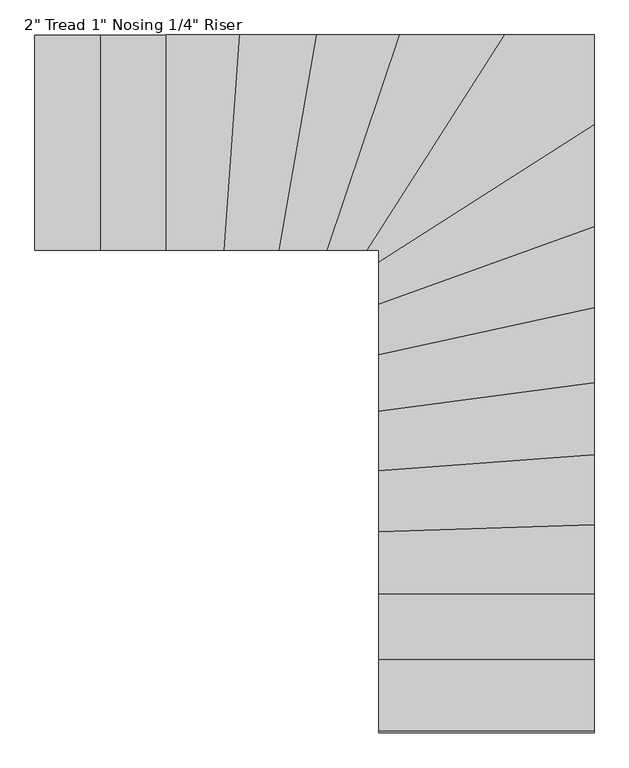
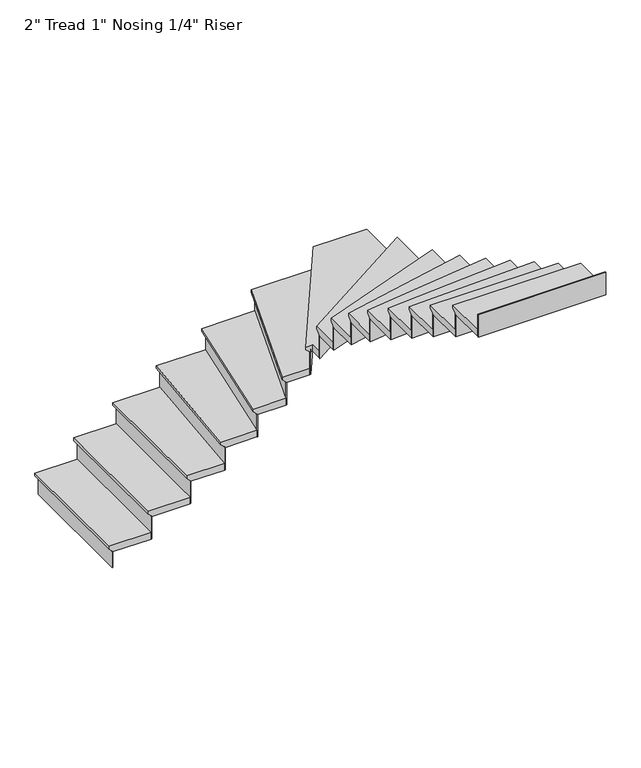
"""IFC4 building model written with IfcOpenShell, lengths in millimetres: stair flight geometry."""

from ifc_helpers import new_model, si_unit, origin, place, context, project, spatial, faceted_brep, source, transform, mapped, element, save


def stair_flight_0e2f916f(model_context):
    return source(origin(), model_context, "Body", "Brep", [
        faceted_brep([(2176.6969821, -801.749605, 488.95), (2176.6969821, -801.749605, 508.0), (2176.6969821, 112.650395, 508.0), (2176.6969821, 112.650395, 488.95), (2202.0969821, -801.749605, 463.55), (2202.0969821, 112.650395, 463.55), (2481.4969821, -801.749605, 508.0), (2481.4969821, 112.650395, 508.0), (2202.0969821, 112.650395, 457.2), (2481.4969821, 112.650395, 457.2), (2481.4969821, -801.749605, 457.2), (2202.0969821, -801.749605, 457.2)], [[[0, 1, 2, 3]], [[4, 0, 3, 5]], [[2, 1, 6, 7]], [[8, 9, 10, 11]], [[2, 7, 9, 8, 5, 3]], [[8, 11, 4, 5]], [[6, 1, 0, 4, 11, 10]], [[7, 6, 10, 9]]]),
        faceted_brep([(2202.0969821, -801.749605, 457.2), (2202.0969821, -801.749605, 338.6666667), (2208.4469821, -801.749605, 338.6666667), (2208.4469821, -801.749605, 457.2), (2202.0969821, 112.650395, 457.2), (2208.4469821, 112.650395, 457.2), (2208.4469821, 112.650395, 338.6666667), (2202.0969821, 112.650395, 338.6666667)], [[[0, 1, 2, 3]], [[4, 5, 6, 7]], [[1, 0, 4, 7]], [[2, 1, 7, 6]], [[3, 2, 6, 5]], [[0, 3, 5, 4]]]),
        faceted_brep([(2481.4969821, -801.749605, 626.5333333), (2481.4969821, -801.749605, 457.2), (2487.8469821, -801.749605, 457.2), (2487.8469821, -801.749605, 626.5333333), (2481.4969821, 112.650395, 626.5333333), (2487.8469821, 112.650395, 626.5333333), (2487.8469821, 112.650395, 457.2), (2481.4969821, 112.650395, 457.2)], [[[0, 1, 2, 3]], [[4, 5, 6, 7]], [[1, 0, 4, 7]], [[2, 1, 7, 6]], [[3, 2, 6, 5]], [[0, 3, 5, 4]]]),
        faceted_brep([(2456.0969821, 112.650395, 677.3333333), (2456.0969821, -801.749605, 677.3333333), (2760.8969821, -801.749605, 677.3333333), (2760.8969821, 112.650395, 677.3333333), (2481.4969821, 112.650395, 626.5333333), (2760.8969821, 112.650395, 626.5333333), (2760.8969821, -801.749605, 626.5333333), (2481.4969821, -801.749605, 626.5333333), (2481.4969821, 112.650395, 632.8833333), (2456.0969821, 112.650395, 658.2833333), (2481.4969821, -801.749605, 632.8833333), (2456.0969821, -801.749605, 658.2833333)], [[[0, 1, 2, 3]], [[4, 5, 6, 7]], [[0, 3, 5, 4, 8, 9]], [[4, 7, 10, 8]], [[2, 1, 11, 10, 7, 6]], [[3, 2, 6, 5]], [[11, 1, 0, 9]], [[10, 11, 9, 8]]]),
        faceted_brep([(2760.8969821, -801.749605, 795.8666667), (2760.8969821, -801.749605, 626.5333333), (2767.2469821, -801.749605, 626.5333333), (2767.2469821, -801.749605, 795.8666667), (2760.8969821, 112.650395, 795.8666667), (2767.2469821, 112.650395, 795.8666667), (2767.2469821, 112.650395, 626.5333333), (2760.8969821, 112.650395, 626.5333333)], [[[0, 1, 2, 3]], [[4, 5, 6, 7]], [[1, 0, 4, 7]], [[2, 1, 7, 6]], [[3, 2, 6, 5]], [[0, 3, 5, 4]]]),
        faceted_brep([(2735.4969821, 112.650395, 846.6666667), (2735.4969821, -801.749605, 846.6666667), (3007.6726348, -801.749605, 846.6666667), (3073.0510102, 112.650395, 846.6666667), (2760.8969821, 112.650395, 795.8666667), (3073.0510102, 112.650395, 795.8666667), (3007.6726348, -801.749605, 795.8666667), (2760.8969821, -801.749605, 795.8666667), (2760.8969821, 112.650395, 802.2166667), (2735.4969821, 112.650395, 827.6166667), (2760.8969821, -801.749605, 802.2166667), (2735.4969821, -801.749605, 827.6166667)], [[[0, 1, 2, 3]], [[4, 5, 6, 7]], [[0, 3, 5, 4, 8, 9]], [[4, 7, 10, 8]], [[2, 1, 11, 10, 7, 6]], [[3, 2, 6, 5]], [[11, 1, 0, 9]], [[10, 11, 9, 8]]]),
        faceted_brep([(3007.6726348, -801.749605, 965.2), (3007.6726348, -801.749605, 795.8666667), (3014.0388449, -801.749605, 795.8666667), (3014.0388449, -801.749605, 965.2), (3073.0510102, 112.650395, 965.2), (3079.4172203, 112.650395, 965.2), (3079.4172203, 112.650395, 795.8666667), (3073.0510102, 112.650395, 795.8666667)], [[[0, 1, 2, 3]], [[4, 5, 6, 7]], [[1, 0, 4, 7]], [[2, 1, 7, 6]], [[3, 2, 6, 5]], [[0, 3, 5, 4]]]),
        faceted_brep([(3047.5861699, 112.650395, 1016.0), (2982.2077944, -801.749605, 1016.0), (3240.3003214, -801.749605, 1016.0), (3399.8612616, 112.650395, 1016.0), (3073.0510102, 112.650395, 965.2), (3399.8612616, 112.650395, 965.2), (3240.3003214, -801.749605, 965.2), (3007.6726348, -801.749605, 965.2), (3073.0510102, 112.650395, 971.55), (3047.5861699, 112.650395, 996.95), (3007.6726348, -801.749605, 971.55), (2982.2077944, -801.749605, 996.95)], [[[0, 1, 2, 3]], [[4, 5, 6, 7]], [[0, 3, 5, 4, 8, 9]], [[4, 7, 10, 8]], [[2, 1, 11, 10, 7, 6]], [[3, 2, 6, 5]], [[11, 1, 0, 9]], [[10, 11, 9, 8]]]),
        faceted_brep([(3240.3003214, -801.749605, 1134.5333333), (3240.3003214, -801.749605, 965.2), (3246.7462737, -801.749605, 965.2), (3246.7462737, -801.749605, 1134.5333333), (3399.8612616, 112.650395, 1134.5333333), (3406.307214, 112.650395, 1134.5333333), (3406.307214, 112.650395, 965.2), (3399.8612616, 112.650395, 965.2)], [[[0, 1, 2, 3]], [[4, 5, 6, 7]], [[1, 0, 4, 7]], [[2, 1, 7, 6]], [[3, 2, 6, 5]], [[0, 3, 5, 4]]]),
        faceted_brep([(3374.0774523, 112.650395, 1185.3333333), (3214.516512, -801.749605, 1185.3333333), (3447.0092595, -801.749605, 1185.3333333), (3753.9707002, 112.650395, 1185.3333333), (3399.8612616, 112.650395, 1134.5333333), (3753.9707002, 112.650395, 1134.5333333), (3447.0092595, -801.749605, 1134.5333333), (3240.3003214, -801.749605, 1134.5333333), (3399.8612616, 112.650395, 1140.8833333), (3374.0774523, 112.650395, 1166.2833333), (3240.3003214, -801.749605, 1140.8833333), (3214.516512, -801.749605, 1166.2833333)], [[[0, 1, 2, 3]], [[4, 5, 6, 7]], [[0, 3, 5, 4, 8, 9]], [[4, 7, 10, 8]], [[2, 1, 11, 10, 7, 6]], [[3, 2, 6, 5]], [[11, 1, 0, 9]], [[10, 11, 9, 8]]]),
        faceted_brep([(3447.0092595, -801.749605, 1303.8666667), (3447.0092595, -801.749605, 1134.5333333), (3453.7075089, -801.749605, 1134.5333333), (3453.7075089, -801.749605, 1303.8666667), (3753.9707002, 112.650395, 1303.8666667), (3760.6689496, 112.650395, 1303.8666667), (3760.6689496, 112.650395, 1134.5333333), (3753.9707002, 112.650395, 1134.5333333)], [[[0, 1, 2, 3]], [[4, 5, 6, 7]], [[1, 0, 4, 7]], [[2, 1, 7, 6]], [[3, 2, 6, 5]], [[0, 3, 5, 4]]]),
        faceted_brep([(3727.1777025, 112.650395, 1354.6666667), (3420.2162618, -801.749605, 1354.6666667), (3618.669605, -801.749605, 1354.6666667), (4203.2690404, 112.650395, 1354.6666667), (3753.9707002, 112.650395, 1303.8666667), (4203.2690404, 112.650395, 1303.8666667), (3618.669605, -801.749605, 1303.8666667), (3447.0092595, -801.749605, 1303.8666667), (3753.9707002, 112.650395, 1310.2166667), (3727.1777025, 112.650395, 1335.6166667), (3447.0092595, -801.749605, 1310.2166667), (3420.2162618, -801.749605, 1335.6166667)], [[[0, 1, 2, 3]], [[4, 5, 6, 7]], [[0, 3, 5, 4, 8, 9]], [[4, 7, 10, 8]], [[2, 1, 11, 10, 7, 6]], [[3, 2, 6, 5]], [[11, 1, 0, 9]], [[10, 11, 9, 8]]]),
        faceted_brep([(3618.669605, -801.749605, 1473.2), (3618.669605, -801.749605, 1303.8666667), (3626.2064355, -801.749605, 1303.8666667), (3626.2064355, -801.749605, 1473.2), (4203.2690404, 112.650395, 1473.2), (4210.8058709, 112.650395, 1473.2), (4210.8058709, 112.650395, 1303.8666667), (4203.2690404, 112.650395, 1303.8666667)], [[[0, 1, 2, 3]], [[4, 5, 6, 7]], [[1, 0, 4, 7]], [[2, 1, 7, 6]], [[3, 2, 6, 5]], [[0, 3, 5, 4]]]),
        faceted_brep([(4553.8339716, -298.2091795, 1524.0), (4553.8339716, 112.650395, 1524.0), (4173.1217188, 112.650395, 1524.0), (3588.5222834, -801.749605, 1524.0), (3639.4339716, -801.749605, 1524.0), (3639.4339716, -882.8086149, 1524.0), (4553.8339716, 112.650395, 1473.2), (4553.8339716, -298.2091795, 1473.2), (3639.4339716, -882.8086149, 1473.2), (3639.4339716, -801.749605, 1473.2), (3618.669605, -801.749605, 1473.2), (4203.2690404, 112.650395, 1473.2), (3618.669605, -801.749605, 1479.55), (4203.2690404, 112.650395, 1479.55), (3588.5222834, -801.749605, 1504.95), (4173.1217188, 112.650395, 1504.95)], [[[0, 1, 2, 3, 4, 5]], [[6, 7, 8, 9, 10, 11]], [[1, 0, 7, 6]], [[11, 10, 12, 13]], [[4, 3, 14, 12, 10, 9]], [[0, 5, 8, 7]], [[14, 3, 2, 15]], [[12, 14, 15, 13]], [[2, 1, 6, 11, 13, 15]], [[5, 4, 9, 8]]]),
        faceted_brep([(3639.4339716, -882.8086149, 1642.5333333), (3639.4339716, -882.8086149, 1473.2), (3639.4339716, -890.3454453, 1473.2), (3639.4339716, -890.3454453, 1642.5333333), (4553.8339716, -298.2091795, 1642.5333333), (4553.8339716, -305.7460099, 1642.5333333), (4553.8339716, -305.7460099, 1473.2), (4553.8339716, -298.2091795, 1473.2)], [[[0, 1, 2, 3]], [[4, 5, 6, 7]], [[1, 0, 4, 7]], [[2, 1, 7, 6]], [[3, 2, 6, 5]], [[0, 3, 5, 4]]]),
        faceted_brep([(4553.8339716, -268.0618578, 1693.3333333), (3639.4339716, -852.6612932, 1693.3333333), (3639.4339716, -1058.7649268, 1693.3333333), (4553.8339716, -730.188422, 1693.3333333), (4553.8339716, -298.2091795, 1642.5333333), (4553.8339716, -730.188422, 1642.5333333), (3639.4339716, -1058.7649268, 1642.5333333), (3639.4339716, -882.8086149, 1642.5333333), (4553.8339716, -298.2091795, 1648.8833333), (4553.8339716, -268.0618578, 1674.2833333), (3639.4339716, -882.8086149, 1648.8833333), (3639.4339716, -852.6612932, 1674.2833333)], [[[0, 1, 2, 3]], [[4, 5, 6, 7]], [[0, 3, 5, 4, 8, 9]], [[4, 7, 10, 8]], [[2, 1, 11, 10, 7, 6]], [[3, 2, 6, 5]], [[11, 1, 0, 9]], [[10, 11, 9, 8]]]),
        faceted_brep([(3639.4339716, -1058.7649268, 1811.8666667), (3639.4339716, -1058.7649268, 1642.5333333), (3639.4339716, -1065.5124468, 1642.5333333), (3639.4339716, -1065.5124468, 1811.8666667), (4553.8339716, -730.188422, 1811.8666667), (4553.8339716, -736.935942, 1811.8666667), (4553.8339716, -736.935942, 1642.5333333), (4553.8339716, -730.188422, 1642.5333333)], [[[0, 1, 2, 3]], [[4, 5, 6, 7]], [[1, 0, 4, 7]], [[2, 1, 7, 6]], [[3, 2, 6, 5]], [[0, 3, 5, 4]]]),
        faceted_brep([(4553.8339716, -703.1983421, 1862.6666667), (3639.4339716, -1031.7748469, 1862.6666667), (3639.4339716, -1272.8813259, 1862.6666667), (4553.8339716, -1072.8926593, 1862.6666667), (4553.8339716, -730.188422, 1811.8666667), (4553.8339716, -1072.8926593, 1811.8666667), (3639.4339716, -1272.8813259, 1811.8666667), (3639.4339716, -1058.7649268, 1811.8666667), (4553.8339716, -730.188422, 1818.2166667), (4553.8339716, -703.1983421, 1843.6166667), (3639.4339716, -1058.7649268, 1818.2166667), (3639.4339716, -1031.7748469, 1843.6166667)], [[[0, 1, 2, 3]], [[4, 5, 6, 7]], [[0, 3, 5, 4, 8, 9]], [[4, 7, 10, 8]], [[2, 1, 11, 10, 7, 6]], [[3, 2, 6, 5]], [[11, 1, 0, 9]], [[10, 11, 9, 8]]]),
        faceted_brep([(3639.4339716, -1272.8813259, 1981.2), (3639.4339716, -1272.8813259, 1811.8666667), (3639.4339716, -1279.3814254, 1811.8666667), (3639.4339716, -1279.3814254, 1981.2), (4553.8339716, -1072.8926593, 1981.2), (4553.8339716, -1079.3927588, 1981.2), (4553.8339716, -1079.3927588, 1811.8666667), (4553.8339716, -1072.8926593, 1811.8666667)], [[[0, 1, 2, 3]], [[4, 5, 6, 7]], [[1, 0, 4, 7]], [[2, 1, 7, 6]], [[3, 2, 6, 5]], [[0, 3, 5, 4]]]),
        faceted_brep([(4553.8339716, -1046.8922612, 2032.0), (3639.4339716, -1246.8809278, 2032.0), (3639.4339716, -1512.428366, 2032.0), (4553.8339716, -1391.3879539, 2032.0), (4553.8339716, -1072.8926593, 1981.2), (4553.8339716, -1391.3879539, 1981.2), (3639.4339716, -1512.428366, 1981.2), (3639.4339716, -1272.8813259, 1981.2), (4553.8339716, -1072.8926593, 1987.55), (4553.8339716, -1046.8922612, 2012.95), (3639.4339716, -1272.8813259, 1987.55), (3639.4339716, -1246.8809278, 2012.95)], [[[0, 1, 2, 3]], [[4, 5, 6, 7]], [[0, 3, 5, 4, 8, 9]], [[4, 7, 10, 8]], [[2, 1, 11, 10, 7, 6]], [[3, 2, 6, 5]], [[11, 1, 0, 9]], [[10, 11, 9, 8]]]),
        faceted_brep([(3639.4339716, -1512.428366, 2150.5333333), (3639.4339716, -1512.428366, 1981.2), (3639.4339716, -1518.8337573, 1981.2), (3639.4339716, -1518.8337573, 2150.5333333), (4553.8339716, -1391.3879539, 2150.5333333), (4553.8339716, -1397.7933452, 2150.5333333), (4553.8339716, -1397.7933452, 1981.2), (4553.8339716, -1391.3879539, 1981.2)], [[[0, 1, 2, 3]], [[4, 5, 6, 7]], [[1, 0, 4, 7]], [[2, 1, 7, 6]], [[3, 2, 6, 5]], [[0, 3, 5, 4]]]),
        faceted_brep([(4553.8339716, -1365.7663885, 2201.3333333), (3639.4339716, -1486.8068005, 2201.3333333), (3639.4339716, -1764.9750907, 2201.3333333), (4553.8339716, -1697.3368865, 2201.3333333), (4553.8339716, -1391.3879539, 2150.5333333), (4553.8339716, -1697.3368865, 2150.5333333), (3639.4339716, -1764.9750907, 2150.5333333), (3639.4339716, -1512.428366, 2150.5333333), (4553.8339716, -1391.3879539, 2156.8833333), (4553.8339716, -1365.7663885, 2182.2833333), (3639.4339716, -1512.428366, 2156.8833333), (3639.4339716, -1486.8068005, 2182.2833333)], [[[0, 1, 2, 3]], [[4, 5, 6, 7]], [[0, 3, 5, 4, 8, 9]], [[4, 7, 10, 8]], [[2, 1, 11, 10, 7, 6]], [[3, 2, 6, 5]], [[11, 1, 0, 9]], [[10, 11, 9, 8]]]),
        faceted_brep([(3639.4339716, -1764.9750907, 2319.8666667), (3639.4339716, -1764.9750907, 2150.5333333), (3639.4339716, -1771.3424392, 2150.5333333), (3639.4339716, -1771.3424392, 2319.8666667), (4553.8339716, -1697.3368865, 2319.8666667), (4553.8339716, -1703.704235, 2319.8666667), (4553.8339716, -1703.704235, 2150.5333333), (4553.8339716, -1697.3368865, 2150.5333333)], [[[0, 1, 2, 3]], [[4, 5, 6, 7]], [[1, 0, 4, 7]], [[2, 1, 7, 6]], [[3, 2, 6, 5]], [[0, 3, 5, 4]]]),
        faceted_brep([(4553.8339716, -1671.8674924, 2370.6666667), (3639.4339716, -1739.5056966, 2370.6666667), (3639.4339716, -2025.0542039, 2370.6666667), (4553.8339716, -1995.9447198, 2370.6666667), (4553.8339716, -1697.3368865, 2319.8666667), (4553.8339716, -1995.9447198, 2319.8666667), (3639.4339716, -2025.0542039, 2319.8666667), (3639.4339716, -1764.9750907, 2319.8666667), (4553.8339716, -1697.3368865, 2326.2166667), (4553.8339716, -1671.8674924, 2351.6166667), (3639.4339716, -1764.9750907, 2326.2166667), (3639.4339716, -1739.5056966, 2351.6166667)], [[[0, 1, 2, 3]], [[4, 5, 6, 7]], [[0, 3, 5, 4, 8, 9]], [[4, 7, 10, 8]], [[2, 1, 11, 10, 7, 6]], [[3, 2, 6, 5]], [[11, 1, 0, 9]], [[10, 11, 9, 8]]]),
        faceted_brep([(3639.4339716, -2025.0542039, 2489.2), (3639.4339716, -2025.0542039, 2319.8666667), (3639.4339716, -2031.4074208, 2319.8666667), (3639.4339716, -2031.4074208, 2489.2), (4553.8339716, -1995.9447198, 2489.2), (4553.8339716, -2002.2979367, 2489.2), (4553.8339716, -2002.2979367, 2319.8666667), (4553.8339716, -1995.9447198, 2319.8666667)], [[[0, 1, 2, 3]], [[4, 5, 6, 7]], [[1, 0, 4, 7]], [[2, 1, 7, 6]], [[3, 2, 6, 5]], [[0, 3, 5, 4]]]),
        faceted_brep([(4553.8339716, -1970.5318524, 2540.0), (3639.4339716, -1999.6413366, 2540.0), (3639.4339716, -2289.8865945, 2540.0), (4553.8339716, -2289.8865945, 2540.0), (4553.8339716, -1995.9447198, 2489.2), (4553.8339716, -2289.8865945, 2489.2), (3639.4339716, -2289.8865945, 2489.2), (3639.4339716, -2025.0542039, 2489.2), (4553.8339716, -1995.9447198, 2495.55), (4553.8339716, -1970.5318524, 2520.95), (3639.4339716, -2025.0542039, 2495.55), (3639.4339716, -1999.6413366, 2520.95)], [[[0, 1, 2, 3]], [[4, 5, 6, 7]], [[0, 3, 5, 4, 8, 9]], [[4, 7, 10, 8]], [[2, 1, 11, 10, 7, 6]], [[3, 2, 6, 5]], [[11, 1, 0, 9]], [[10, 11, 9, 8]]]),
        faceted_brep([(3639.4339716, -2289.8865945, 2658.5333333), (3639.4339716, -2289.8865945, 2489.2), (3639.4339716, -2296.2365945, 2489.2), (3639.4339716, -2296.2365945, 2658.5333333), (4553.8339716, -2289.8865945, 2658.5333333), (4553.8339716, -2296.2365945, 2658.5333333), (4553.8339716, -2296.2365945, 2489.2), (4553.8339716, -2289.8865945, 2489.2)], [[[0, 1, 2, 3]], [[4, 5, 6, 7]], [[1, 0, 4, 7]], [[2, 1, 7, 6]], [[3, 2, 6, 5]], [[0, 3, 5, 4]]]),
        faceted_brep([(4553.8339716, -2264.4865945, 2709.3333333), (3639.4339716, -2264.4865945, 2709.3333333), (3639.4339716, -2569.2865945, 2709.3333333), (4553.8339716, -2569.2865945, 2709.3333333), (4553.8339716, -2289.8865945, 2658.5333333), (4553.8339716, -2569.2865945, 2658.5333333), (3639.4339716, -2569.2865945, 2658.5333333), (3639.4339716, -2289.8865945, 2658.5333333), (4553.8339716, -2289.8865945, 2664.8833333), (4553.8339716, -2264.4865945, 2690.2833333), (3639.4339716, -2289.8865945, 2664.8833333), (3639.4339716, -2264.4865945, 2690.2833333)], [[[0, 1, 2, 3]], [[4, 5, 6, 7]], [[0, 3, 5, 4, 8, 9]], [[4, 7, 10, 8]], [[2, 1, 11, 10, 7, 6]], [[3, 2, 6, 5]], [[11, 1, 0, 9]], [[10, 11, 9, 8]]]),
        faceted_brep([(3639.4339716, -2569.2865945, 2827.8666667), (3639.4339716, -2569.2865945, 2658.5333333), (3639.4339716, -2575.6365945, 2658.5333333), (3639.4339716, -2575.6365945, 2827.8666667), (4553.8339716, -2569.2865945, 2827.8666667), (4553.8339716, -2575.6365945, 2827.8666667), (4553.8339716, -2575.6365945, 2658.5333333), (4553.8339716, -2569.2865945, 2658.5333333)], [[[0, 1, 2, 3]], [[4, 5, 6, 7]], [[1, 0, 4, 7]], [[2, 1, 7, 6]], [[3, 2, 6, 5]], [[0, 3, 5, 4]]]),
        faceted_brep([(3639.4339716, -2848.6865945, 2997.2), (3639.4339716, -2848.6865945, 2827.8666667), (3639.4339716, -2855.0365945, 2827.8666667), (3639.4339716, -2855.0365945, 2997.2), (4553.8339716, -2848.6865945, 2997.2), (4553.8339716, -2855.0365945, 2997.2), (4553.8339716, -2855.0365945, 2827.8666667), (4553.8339716, -2848.6865945, 2827.8666667)], [[[0, 1, 2, 3]], [[4, 5, 6, 7]], [[1, 0, 4, 7]], [[2, 1, 7, 6]], [[3, 2, 6, 5]], [[0, 3, 5, 4]]]),
        faceted_brep([(4553.8339716, -2543.8865945, 2878.6666667), (3639.4339716, -2543.8865945, 2878.6666667), (3639.4339716, -2848.6865945, 2878.6666667), (4553.8339716, -2848.6865945, 2878.6666667), (4553.8339716, -2569.2865945, 2827.8666667), (4553.8339716, -2848.6865945, 2827.8666667), (3639.4339716, -2848.6865945, 2827.8666667), (3639.4339716, -2569.2865945, 2827.8666667), (4553.8339716, -2569.2865945, 2834.2166667), (4553.8339716, -2543.8865945, 2859.6166667), (3639.4339716, -2569.2865945, 2834.2166667), (3639.4339716, -2543.8865945, 2859.6166667)], [[[0, 1, 2, 3]], [[4, 5, 6, 7]], [[0, 3, 5, 4, 8, 9]], [[4, 7, 10, 8]], [[2, 1, 11, 10, 7, 6]], [[3, 2, 6, 5]], [[11, 1, 0, 9]], [[10, 11, 9, 8]]]),
    ])


if __name__ == "__main__":
    model = new_model("IFC4")
    model_context = context("Model", 3, world=origin())
    ifc_project = project(units=[si_unit("LENGTHUNIT", "METRE", prefix="MILLI")], contexts=[model_context])
    site = spatial("IfcSite", under=ifc_project)
    building = spatial("IfcBuilding", under=site)
    placement = place(None, origin())
    stair_flight_shape = stair_flight_0e2f916f(model_context)
    element("IfcStairFlight", 1, ObjectType="2\" Tread 1\" Nosing 1/4\" Riser", at=placement, inside=building, context=model_context, shape_type="MappedRepresentation", body=[
        mapped(stair_flight_shape, transform((0.0, 0.0, 0.0), x_axis=(1.0, 0.0, 0.0), y_axis=(0.0, 1.0, 0.0), z_axis=(0.0, 0.0, 1.0))),
    ])
    save(model, "model.ifc")
